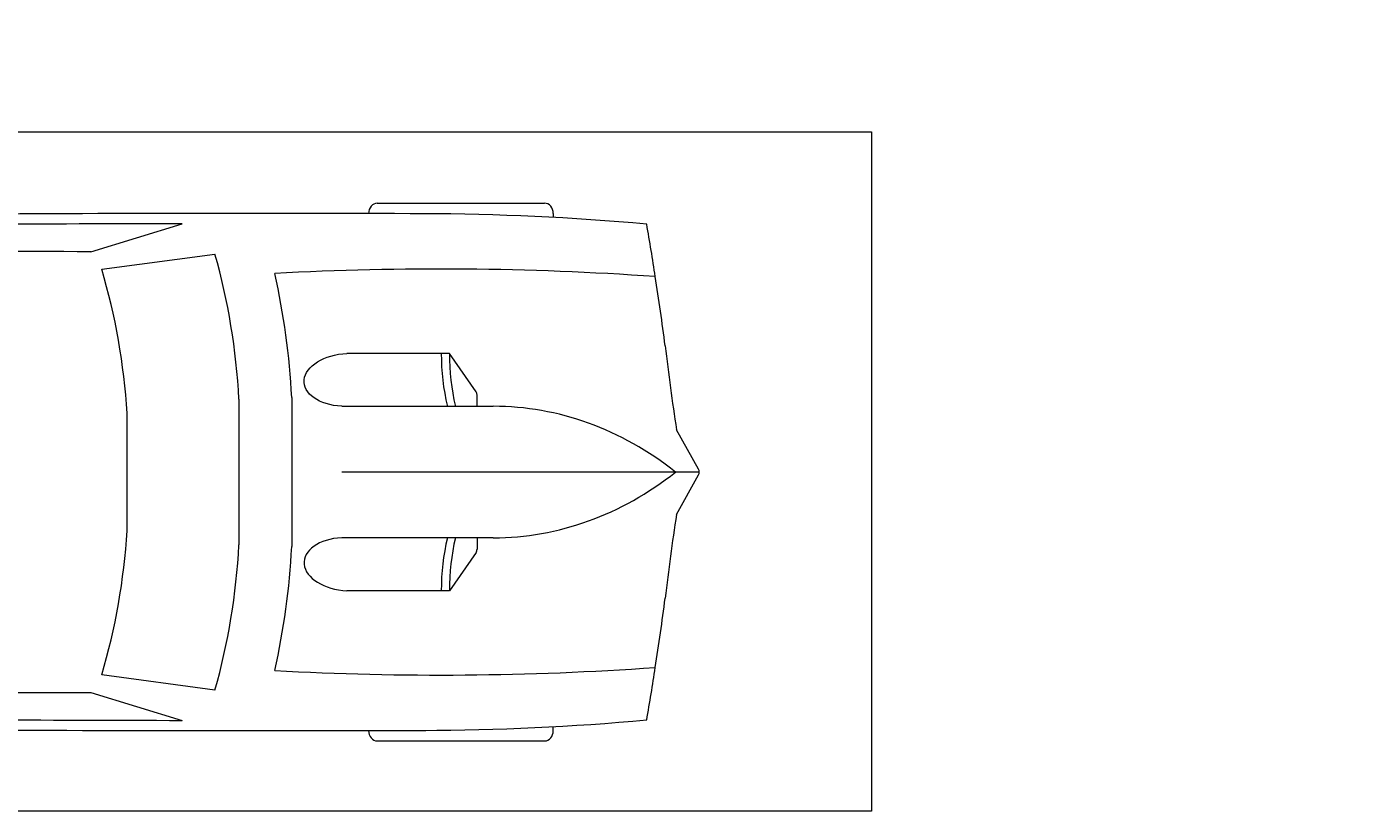
# Model space of a CAD drawing. Units: inches. Extents: x -46 to 1145, y -527 to 760.
# Tile 12 of 57: x 380 to 573, y -270 to -157. Entities that reach past the tile are written whole.
import ezdxf

# ---------------------------------------------------------------- set-up
doc = ezdxf.new("R2010")
doc.units = ezdxf.units.IN
doc.header["$MEASUREMENT"] = 0
for name, color, linetype, lineweight in [('A-ANNO-DIMS', 2, 'Continuous', 18), ('C-PKNG', 8, 'Continuous', 18), ('C-PKNG-VEHI', 8, 'Continuous', 13)]:
    doc.layers.add(name, color=color, linetype=linetype, lineweight=lineweight)
doc.styles.get("Standard").update_dxf_attribs({"font": 'arial.ttf'})
doc.dimstyles.get("Standard").update_dxf_attribs({"dimtxt": 0.18, "dimasz": 0.18, "dimexe": 0.18, "dimexo": 0.0625, "dimgap": 0.09, "dimtad": 0, "dimtih": 1, "dimtoh": 1, "dimdec": 0, "dimzin": 0, "dimdsep": 46, "dimlunit": 3, "dimtxsty": 'Standard', "dimcen": 0.09, "dimadec": 0, "dimazin": 0, "dimtfac": 1, "dimtdec": 0, "dimtofl": 0, "dimtmove": 0, "dimatfit": 3, "dimfxl": 1, "dimtolj": 1, "dimtzin": 0, "dimarcsym": 0})

# ---------------------------------------------------------------- blocks, each defined once
blk = doc.blocks.new('*U640')
for p, q in [((1182.5, 987.8), (567.7, 987.8)), ((3472.1, 987.8), (4086.9, 987.8)), ((536, 950.2), (536, 935.5)), ((1214.1, 949.7), (1214.1, 950.2)), ((3440.5, 941.7), (3440.5, 950.2)), ((4118.5, 950.2), (4118.5, 934.1)), ((2234.8, 809.5), (1898.9, 912.4)), ((3411.6, 904.3), (3029.9, 807.2)), ((4736.4, -850.9), (4736.4, 850.9)), ((1778.8, 801), (2194.7, 745.5)), ((4785.3, -832.1), (4785.3, 832.1)), ((3515.9, 745.5), (3994.1, 745.5)), ((4736.4, 745.5), (4242, 745.5)), ((4178.7, 670.3), (4178.7, -670.3)), ((819.6, 295.3), (917.7, 436.1)), ((917.7, 436.1), (1293.8, 436.1)), ((815.9, 241.4), (815.9, 283.3)), ((1496.5, -273.7), (1496.5, 273.7)), ((1690.4, -267.4), (1690.4, 267.4)), ((4736.4, -267.4), (4736.4, 267.4)), ((756.2, 241.4), (1312.8, 241.4)), ((2101.5, 215.8), (2101.5, -215.8)), ((83, 155.7), (2.6, 10.3)), ((0, 0), (1312.8, 0)), ((2.6, -10.3), (83, -155.7)), ((756.2, -241.4), (1312.8, -241.4)), ((815.9, -241.4), (815.9, -283.3)), ((819.6, -295.3), (917.7, -436.1)), ((917.7, -436.1), (1293.8, -436.1)), ((2194.7, -745.5), (1778.8, -801)), ((3994.1, -745.5), (3515.9, -745.5)), ((4242, -745.5), (4736.4, -745.5)), ((2234.8, -809.5), (1898.9, -912.4)), ((3411.6, -904.3), (3029.9, -807.2)), ((536, -950.2), (536, -935.5)), ((1214.1, -949.7), (1214.1, -950.2)), ((3440.5, -941.7), (3440.5, -950.2)), ((4118.5, -950.2), (4118.5, -934.1)), ((1182.5, -987.8), (567.7, -987.8)), ((3472.1, -987.8), (4086.9, -987.8))]:
    blk.add_line(p, q)
for centre, major_axis, ratio, start_param, end_param in [((567.7, 950.2), (0, -37.6), 0.842304, 3.141593, 4.712389), ((1182.5, 950.2), (0, 37.6), 0.842304, -1.570796, 0), ((3472.1, 950.2), (0, -37.6), 0.842304, 3.141593, 4.712389), ((4086.9, 950.2), (0, 37.6), 0.842304, -1.570796, 0), ((1046.3, -12467.9), (0, 13417.1), 0.842304, 0.00281, 0.075598), ((1637.8, -268112.7), (0, 269062.9), 0.842304, -0.013397, 0.002797), ((4588, 910.3), (0, 56.4), 0.842304, -0.013017, 1.249894), ((1637.8, -268131.5), (0, 269121), 0.842304, -0.013397, -0.013017), ((4673.1, 832.1), (0, -133.3), 0.842304, 1.570796, 3.128196), ((6757.2, -699.1), (0, 7958), 0.842304, 1.367076, 1.39176), ((1637.8, -268112.7), (0, -269025.3), 0.842304, 3.133765, 3.140441), ((4673.1, 850.9), (0, -75.2), 0.842304, 1.570796, 3.128196), ((3436.4, 136.8), (0, 2077), 0.842304, 1.245306, 1.50788), ((2433, -93125.4), (0, -93935.2), 0.842304, 3.134049, 3.144098), ((951.8, -15086.6), (0, -15832.5), 0.842304, 3.096046, 3.200911), ((3799.7, 71.1), (0, -2021.3), 0.842304, 4.372215, 4.640744), ((433.9, 0), (0, 3734.3), 0.842304, 4.511394, 4.913384), ((912, 0), (0, 3734.3), 0.842304, 4.511394, 4.913384), ((4242, 670.3), (0, 75.2), 0.842304, 0, 1.570796), ((6583, -699.1), (0, -7754.7), 0.842304, 4.528606, 4.561838), ((3413.8, 136.8), (0, -2280.3), 0.842304, 4.449482, 4.652344), ((-5194.2, 1330.9), (0, -6374.4), 0.842304, 1.385369, 1.434372), ((331.1, 432), (0, 696.4), 0.842304, 4.435146, 4.718221), ((360.7, 432), (0, 696.4), 0.842304, 4.435146, 4.718221), ((1290.1, 338.8), (161, -9.1), 0.603834, -1.395552, 1.581315), ((831.8, 283.3), (0, 18.8), 0.842304, 0.879714, 1.570796), ((756.2, -1185.2), (0, 1426.7), 0.842304, 0, 0.590319), ((15.8, 0), (0, -18.8), 0.842304, 4.131459, 5.293319), ((756.2, 1185.2), (0, 1426.7), 0.842304, 2.551274, 3.141593), ((-5194.2, -1330.9), (0, 6374.4), 0.842304, -1.434372, -1.385369), ((331.1, -432), (0, -696.4), 0.842304, 1.564964, 1.848039), ((360.7, -432), (0, -696.4), 0.842304, 1.564964, 1.848039), ((3799.7, -71.1), (0, -2021.3), 0.842304, -1.499151, -1.230623), ((831.8, -283.3), (0, -18.8), 0.842304, 4.712389, 5.403472), ((3413.8, -136.8), (0, -2280.3), 0.842304, -1.510751, -1.307889), ((3436.4, -136.8), (0, -2077), 0.842304, -1.50788, -1.245306), ((6583, 699.1), (0, 7754.7), 0.842304, 1.721348, 1.754579), ((4242, -670.3), (0, -75.2), 0.842304, 4.712389, 6.283185), ((6757.2, 699.1), (0, 7958), 0.842304, 1.749832, 1.774517), ((951.8, 15086.6), (0, -15832.5), 0.842304, -0.059319, 0.045547), ((2433, 93125.4), (0, -93935.2), 0.842304, -0.002505, 0.007544), ((4673.1, -832.1), (0, -133.3), 0.842304, 0.013397, 1.570796), ((4673.1, -850.9), (0, 75.2), 0.842304, 3.15499, 4.712389), ((1046.3, 12467.9), (0, -13417.1), 0.842304, -0.075598, -0.00281), ((1637.8, 268112.7), (0, 269062.9), 0.842304, 3.138796, 3.15499), ((1637.8, 268112.7), (0, -269025.3), 0.842304, 0.001152, 0.007828), ((4588, -910.3), (0, -56.4), 0.842304, -1.249894, 0.013017), ((567.7, -950.2), (0, 37.6), 0.842304, 1.570796, 3.141593), ((1182.5, -950.2), (0, -37.6), 0.842304, 0, 1.570796), ((3472.1, -950.2), (0, -37.6), 0.842304, -1.570796, 0), ((4086.9, -950.2), (0, 37.6), 0.842304, 3.141593, 4.712389), ((1637.8, 268131.5), (0, 269121), 0.842304, 3.15461, 3.15499)]:
    blk.add_ellipse(centre, major_axis=major_axis, ratio=ratio, start_param=start_param, end_param=end_param)
at = {"extrusion": (0, 0, -1)}
blk.add_ellipse((1290.1, -338.8), major_axis=(161, 9.1), ratio=0.603834, start_param=-1.395552, end_param=1.581315, dxfattribs=at)
blk = doc.blocks.new('*D702')
at = {"layer": 'A-ANNO-DIMS', "color": 0, "lineweight": -2, "transparency": 16777216}
for p, q in [((189.63, -39.48), (1145.34, -39.48)), ((1145.16, -39.66), (1145.16, -249.3)), ((1145.16, -459.3), (1145.16, -249.66)), ((183.63, -459.48), (1145.34, -459.48))]:
    blk.add_line(p, q, dxfattribs=at)
at = {"layer": 'A-ANNO-DIMS', "color": 0, "transparency": 16777216}
for points in [[(1145.13, -39.66), (1145.19, -39.66), (1145.16, -39.48)], [(1145.13, -459.3), (1145.19, -459.3), (1145.16, -459.48)]]:
    blk.add_solid(points, dxfattribs=at)
at = {"layer": 'Defpoints', "color": 0, "transparency": 16777216}
for p in [(189.56, -39.48), (1145.16, -39.48), (183.56, -459.48)]:
    blk.add_point(p, dxfattribs=at)
at = {"layer": 'A-ANNO-DIMS', "color": 0, "transparency": 16777216, "insert": (1145.16, -249.48), "char_height": 0.18, "attachment_point": 5}
blk.add_mtext('\\A1;420', dxfattribs=at)

msp = doc.modelspace()

# ---------------------------------------------------------------- linework, layer by layer
at = {"layer": 'C-PKNG'}
msp.add_lwpolyline([(501.7297, -270.4792), (273.5156, -270.4792), (273.5156, -172.1813), (501.7297, -172.1813)], close=True, dxfattribs=at)

# ---------------------------------------------------------------- block references
at = {"layer": 'C-PKNG-VEHI', "xscale": 0.0393700787401575, "yscale": 0.0393700787401575, "zscale": 0.0393700787401575, "rotation": 180}
msp.add_blockref('*U640', (476.808, -221.4019), dxfattribs=at)

# ---------------------------------------------------------------- dimensions: what is measured, and where the dimension line sits
at = {"layer": 'A-ANNO-DIMS'}
dim = msp.add_linear_dim(base=(1145.1637, -39.4824), p1=(183.5637, -459.4824), p2=(189.5637, -39.4824), angle=90, dimstyle='Standard', override={"dimdec": 0, "dimlfac": 1, "dimrnd": 0, "dimzin": 0, "dimdsep": 46, "dimlunit": 2}, dxfattribs=at)
dim.commit()
dim.dimension.update_dxf_attribs({"geometry": '*D702', "text_midpoint": (1145.1637, -249.4824)})

doc.saveas('drawing.dxf')
